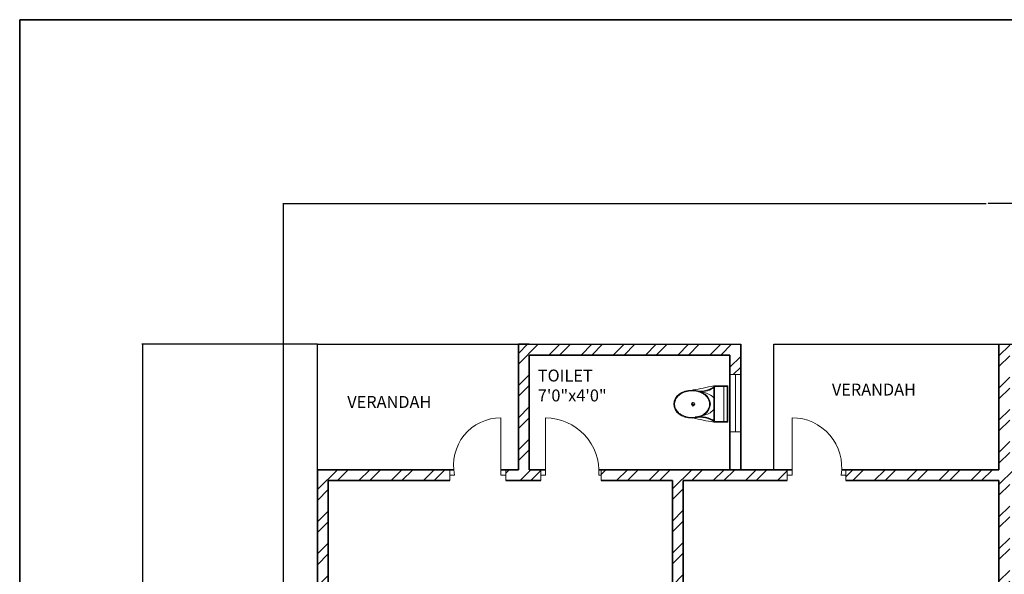
# Model space of a CAD drawing. Units: inches. Extents: x 1962 to 2771, y 1245 to 2660.
# Tile 109 of 114: x 1962 to 2374, y 2428 to 2660. Entities that reach past the tile are written whole.
import ezdxf

# ---------------------------------------------------------------- set-up
doc = ezdxf.new("R2010")
doc.units = ezdxf.units.IN
for name, color, linetype, lineweight in [('A-ANNO-DIMS', 2, 'Continuous', 18), ('A-ANNO-TTLB', 7, 'Continuous', 35), ('A-AREA-IDEN', 7, 'Continuous', 18), ('A-DOOR', 3, 'Continuous', 18), ('A-FLOR-BALC', 7, 'Continuous', 25), ('A-FLOR-FIXT', 8, 'Continuous', 18), ('A-GLAZ', 4, 'Continuous', 18), ('A-WALL', 7, 'Continuous', 35), ('A-WALL-PATT', 252, 'Continuous', 13)]:
    doc.layers.add(name, color=color, linetype=linetype, lineweight=lineweight)
doc.styles.get("Standard").update_dxf_attribs({"font": 'arial.ttf'})
doc.dimstyles.get("Standard").update_dxf_attribs({"dimtxt": 0.18, "dimasz": 0.18, "dimexe": 0.18, "dimexo": 0.0625, "dimgap": 0.09, "dimtad": 0, "dimtih": 1, "dimtoh": 1, "dimdec": 4, "dimzin": 0, "dimdsep": 46, "dimtxsty": 'Standard', "dimcen": 0.09, "dimadec": 0, "dimazin": 0, "dimtfac": 1, "dimtdec": 4, "dimtofl": 0, "dimtmove": 0, "dimatfit": 3, "dimfxl": 1, "dimtolj": 1, "dimtzin": 0, "dimarcsym": 0})

# ---------------------------------------------------------------- blocks, each defined once
blk = doc.blocks.new('A$C31115884')
for p, q in [((283, 498), (223, 498)), ((258, 466), (258, 523)), ((0, 200), (0, 0)), ((520, 200), (0, 200)), ((10, 190), (10, 10)), ((510, 190), (10, 190)), ((510, 10), (510, 190)), ((520, 0), (520, 200)), ((510, 54), (0, 54)), ((10, 10), (510, 10)), ((0, 0), (520, 0))]:
    blk.add_line(p, q)
blk.add_circle((256, 496), 23.6)
for centre, radius, start, end in [((2778, -205), 2807, 165.4549, 171.7133), ((-295, 403), 365, 324.2091, 9.3499), ((-295, 403), 375, 324.2091, 9.3499), ((806, 403), 365, 170.6501, 215.7909), ((3237, 905), 2807, 188.2867, 194.5451), ((384, 406), 293, 190.2774, 224.1564), ((139, 406), 293, 315.8436, 2.6563), ((806, 403), 375, 179.2036, 215.7909)]:
    blk.add_arc(centre, radius, start, end)
blk.add_ellipse((256, 510), major_axis=(0, -261), ratio=0.772727)
blk.add_open_spline([(256, 259), (263, 259), (270, 260), (288, 262), (299, 265), (320, 273), (330, 278), (350, 291), (360, 299), (378, 316), (386, 326), (402, 347), (409, 358), (421, 383), (427, 395), (436, 422), (440, 436), (445, 465), (447, 480), (448, 509), (448, 524), (445, 553), (443, 568), (436, 596), (432, 610), (422, 636), (416, 649), (402, 672), (395, 683), (379, 703), (370, 712), (351, 728), (341, 735), (321, 746), (310, 751), (289, 757), (278, 759), (256, 761), (245, 761), (223, 757), (212, 754), (191, 746), (181, 741), (161, 728), (151, 720), (133, 703), (125, 693), (110, 672), (103, 660), (90, 636), (85, 623), (76, 596), (72, 582), (67, 553), (66, 538), (64, 509), (65, 494), (68, 465), (70, 450), (77, 422), (81, 408), (91, 382), (97, 370), (111, 346), (118, 335), (135, 316), (144, 307), (162, 291), (172, 284), (193, 273), (203, 269), (225, 262), (236, 260), (250, 259), (253, 259), (256, 259)], degree=3, knots=[0, 0, 0, 0, 0.110105, 0.110105, 0.285049, 0.285049, 0.459994, 0.459994, 0.634938, 0.634938, 0.809882, 0.809882, 0.984827, 0.984827, 1.159771, 1.159771, 1.334715, 1.334715, 1.50966, 1.50966, 1.684604, 1.684604, 1.859549, 1.859549, 2.034493, 2.034493, 2.209437, 2.209437, 2.384382, 2.384382, 2.559326, 2.559326, 2.73427, 2.73427, 2.909215, 2.909215, 3.084159, 3.084159, 3.259103, 3.259103, 3.434048, 3.434048, 3.608992, 3.608992, 3.783936, 3.783936, 3.958881, 3.958881, 4.133825, 4.133825, 4.30877, 4.30877, 4.483714, 4.483714, 4.658658, 4.658658, 4.833603, 4.833603, 5.008547, 5.008547, 5.183491, 5.183491, 5.358436, 5.358436, 5.53338, 5.53338, 5.708324, 5.708324, 5.883269, 5.883269, 6.058213, 6.058213, 6.233158, 6.233158, 6.283185, 6.283185, 6.283185, 6.283185])
blk = doc.blocks.new('WIN-24IN-B')
for p, q in [((0, 24), (4.5, 24)), ((4.5, 24), (2.25, 24)), ((2.25, 24), (2.25, 0)), ((4.5, 0), (0, 0)), ((2.25, 0), (4.5, 0))]:
    blk.add_line(p, q)
blk = doc.blocks.new('*D40')
at = {"layer": 'A-ANNO-DIMS', "color": 0, "lineweight": -2, "transparency": 16777216}
for p, q in [((2072.02, 2033.91), (2072.02, 2583.47)), ((2072.2, 2583.29), (2366.02, 2583.29)), ((2660.63, 2583.29), (2366.81, 2583.29)), ((2660.81, 2524.41), (2660.81, 2583.47))]:
    blk.add_line(p, q, dxfattribs=at)
at = {"layer": 'A-ANNO-DIMS', "color": 0, "transparency": 16777216}
for points in [[(2072.2, 2583.32), (2072.2, 2583.26), (2072.02, 2583.29)], [(2660.63, 2583.32), (2660.63, 2583.26), (2660.81, 2583.29)]]:
    blk.add_solid(points, dxfattribs=at)
at = {"layer": 'Defpoints', "color": 0, "transparency": 16777216}
for p in [(2660.81, 2583.29), (2660.81, 2524.34), (2072.02, 2033.84)]:
    blk.add_point(p, dxfattribs=at)
at = {"layer": 'A-ANNO-DIMS', "color": 0, "transparency": 16777216, "insert": (2366.41, 2583.29), "char_height": 0.18, "attachment_point": 5}
blk.add_mtext('\\A1;588.8', dxfattribs=at)
blk = doc.blocks.new('*D43')
at = {"layer": 'A-ANNO-DIMS', "color": 0, "lineweight": -2, "transparency": 16777216}
for p, q in [((2086.24, 2524.34), (2012.89, 2524.34)), ((2013.07, 2524.16), (2013.07, 2279.28)), ((2013.07, 2034.02), (2013.07, 2278.91)), ((2071.96, 2033.84), (2012.89, 2033.84))]:
    blk.add_line(p, q, dxfattribs=at)
at = {"layer": 'A-ANNO-DIMS', "color": 0, "transparency": 16777216}
for points in [[(2013.04, 2524.16), (2013.1, 2524.16), (2013.07, 2524.34)], [(2013.04, 2034.02), (2013.1, 2034.02), (2013.07, 2033.84)]]:
    blk.add_solid(points, dxfattribs=at)
at = {"layer": 'Defpoints', "color": 0, "transparency": 16777216}
for p in [(2086.31, 2524.34), (2013.07, 2033.84), (2072.02, 2033.84)]:
    blk.add_point(p, dxfattribs=at)
at = {"layer": 'A-ANNO-DIMS', "color": 0, "transparency": 16777216, "insert": (2013.07, 2279.09), "char_height": 0.18, "attachment_point": 5}
blk.add_mtext('\\A1;490.5', dxfattribs=at)

msp = doc.modelspace()

# ---------------------------------------------------------------- hatches: boundary and pattern name
at = {"layer": 'A-WALL-PATT'}
h = msp.add_hatch(dxfattribs=at)
h.set_pattern_fill('ANSI32', color=256)
h.paths.add_polyline_path([(2090.8074, 2467.3437), (2141.6481, 2467.3437), (2141.6481, 2469.5937), (2141.6481, 2471.8437), (2086.3074, 2471.8437), (2086.3074, 2422.5333), (2090.8074, 2422.5333)])
h.paths.add_polyline_path([(2282.7664, 2471.8437), (2204.8982, 2471.8437), (2204.8982, 2467.3437), (2234.8074, 2467.3437), (2234.8074, 2311.3437), (2228.7492, 2311.3437), (2228.7492, 2306.8437), (2234.8074, 2306.8437), (2331.9227, 2306.8437), (2331.9227, 2309.0937), (2331.9227, 2311.3437), (2239.3074, 2311.3437), (2239.3074, 2467.3437), (2282.7664, 2467.3437), (2282.7664, 2469.5937)])
h.paths.add_polyline_path([(2471.4531, 2519.8437), (2552.011, 2519.8437), (2564.3996, 2519.8437), (2564.3996, 2511.1389), (2568.8996, 2511.1389), (2568.8996, 2524.3437), (2466.9531, 2524.3437), (2466.9531, 2471.8437), (2450.0749, 2471.8437), (2446.4672, 2471.8437), (2446.4672, 2467.3437), (2450.0749, 2467.3437), (2475.9988, 2467.3437), (2475.9988, 2469.5937), (2475.9988, 2471.8437), (2471.4531, 2471.8437)])
h.paths.add_polyline_path([(2575.2231, 2469.5937), (2575.2231, 2471.8437), (2568.8996, 2471.8437), (2568.8996, 2487.1389), (2564.3996, 2487.1389), (2564.3996, 2471.8437), (2556.511, 2471.8437), (2499.2904, 2471.8437), (2499.2904, 2467.3437), (2507.8074, 2467.3437), (2507.8074, 2311.3437), (2414.863, 2311.3437), (2414.863, 2306.8437), (2512.3074, 2306.8437), (2517.0114, 2306.8437), (2517.0114, 2309.0937), (2517.0114, 2311.3437), (2512.3074, 2311.3437), (2512.3074, 2467.3437), (2575.2231, 2467.3437)])
h.paths.add_polyline_path([(2660.8074, 2471.8437), (2600.9602, 2471.8437), (2600.9602, 2467.3437), (2656.3074, 2467.3437), (2656.3074, 2432.5704), (2660.8074, 2432.5704)])
h.paths.add_polyline_path([(2660.8074, 2372.5704), (2656.3074, 2372.5704), (2656.3074, 2311.3437), (2600.276, 2311.3437), (2600.276, 2309.0937), (2600.276, 2306.8437), (2656.3074, 2306.8437), (2656.3074, 2296.2593), (2660.8074, 2296.2593)])
h.paths.add_polyline_path([(2572.3074, 2306.8437), (2577.1385, 2306.8437), (2577.1385, 2311.3437), (2551.082, 2311.3437), (2551.082, 2306.8437), (2567.8074, 2306.8437), (2567.8074, 2258.8437), (2540.0574, 2258.8437), (2540.0574, 2256.5937), (2540.0574, 2254.3437), (2567.8074, 2254.3437), (2656.3074, 2254.3437), (2656.3074, 2236.9085), (2660.8074, 2236.9085), (2660.8074, 2272.2593), (2656.3074, 2272.2593), (2656.3074, 2258.8437), (2572.3074, 2258.8437)])
h.paths.add_polyline_path([(2512.3074, 2254.3437), (2518.8716, 2254.3437), (2518.8716, 2256.5937), (2518.8716, 2258.8437), (2507.8074, 2258.8437), (2507.8074, 2177.8437), (2567.8074, 2177.8437), (2567.8074, 2172.9628), (2572.3074, 2172.9628), (2572.3074, 2177.8437), (2656.3074, 2177.8437), (2656.3074, 2166.4846), (2660.8074, 2166.4846), (2660.8074, 2200.9085), (2656.3074, 2200.9085), (2656.3074, 2182.3437), (2512.3074, 2182.3437)])
h.paths.add_polyline_path([(2656.3074, 2129.8437), (2572.3074, 2129.8437), (2572.3074, 2150.3044), (2570.0574, 2150.3044), (2567.8074, 2150.3044), (2567.8074, 2129.8437), (2507.8074, 2129.8437), (2507.8074, 2116.3027), (2510.0574, 2116.3027), (2512.3074, 2116.3027), (2512.3074, 2125.3437), (2567.8074, 2125.3437), (2572.3074, 2125.3437), (2656.3074, 2125.3437)])
h.paths.add_polyline_path([(2090.8074, 2362.5333), (2086.3074, 2362.5333), (2086.3074, 2298.6242), (2090.8074, 2298.6242), (2090.8074, 2306.8437), (2174.8074, 2306.8437), (2174.8074, 2286.4178), (2179.3074, 2286.4178), (2179.3074, 2306.8437), (2192.8641, 2306.8437), (2192.8641, 2309.0937), (2192.8641, 2311.3437), (2090.8074, 2311.3437)])
h.paths.add_polyline_path([(2209.156, 2258.8437), (2179.3074, 2258.8437), (2179.3074, 2263.2236), (2177.0574, 2263.2236), (2174.8074, 2263.2236), (2174.8074, 2258.8437), (2090.8074, 2258.8437), (2090.8074, 2274.6242), (2086.3074, 2274.6242), (2086.3074, 2238.2967), (2088.5574, 2238.2967), (2090.8074, 2238.2967), (2090.8074, 2254.3437), (2209.156, 2254.3437)])
h.paths.add_polyline_path([(2090.8074, 2177.8437), (2234.8074, 2177.8437), (2234.8074, 2173.1428), (2239.3074, 2173.1428), (2239.3074, 2258.8437), (2230.8442, 2258.8437), (2230.8442, 2256.5937), (2230.8442, 2254.3437), (2234.8074, 2254.3437), (2234.8074, 2182.3437), (2090.8074, 2182.3437), (2090.8074, 2202.2967), (2086.3074, 2202.2967), (2086.3074, 2140.0389), (2090.8074, 2140.0389)])
h.paths.add_polyline_path([(2090.8074, 2080.0389), (2086.3074, 2080.0389), (2086.3074, 2033.8437), (2090.8074, 2033.8437)], flags=17)
h.paths.add_polyline_path([(2244.9405, 2033.8437), (2239.3074, 2033.8437), (2239.3074, 2142.0665), (2237.2592, 2142.0665), (2234.8074, 2142.0665), (2234.8074, 2033.8437), (2090.8074, 2033.8437), (2076.5204, 2033.8437), (2072.0204, 2033.8437), (2072.0204, 2000.4493), (2076.5204, 2000.4493), (2076.5204, 2029.3437), (2090.8074, 2029.3437), (2244.9405, 2029.3437), (2244.9405, 2031.5937)])
h.paths.add_polyline_path([(2234.8074, 1933.3437), (2076.5204, 1933.3437), (2076.5204, 1952.4493), (2074.2704, 1952.4493), (2072.0204, 1952.4493), (2072.0204, 1933.3437), (2072.0204, 1928.8437), (2234.8074, 1928.8437)])
h.paths.add_polyline_path([(2090.8074, 1928.8437), (2086.3074, 1928.8437), (2086.3074, 1906.5013), (2090.8074, 1906.5013)])
h.paths.add_polyline_path([(2090.8074, 1846.5013), (2086.3074, 1846.5013), (2086.3074, 1769.9917), (2088.5574, 1769.9917), (2090.8074, 1769.9917), (2090.8074, 1780.3437), (2234.8074, 1780.3437), (2234.8074, 1708.3437), (2230.3764, 1708.3437), (2230.3764, 1703.8437), (2239.3074, 1703.8437), (2239.3074, 1792.6669), (2237.0574, 1792.6669), (2234.8074, 1792.6669), (2234.8074, 1784.8437), (2090.8074, 1784.8437)])
h.paths.add_polyline_path([(2239.3074, 1928.8437), (2244.9405, 1928.8437), (2244.9405, 1931.0937), (2244.9405, 1933.3437), (2234.8074, 1933.3437), (2234.8074, 1928.8437), (2234.8074, 1825.5949), (2239.3074, 1825.5949)])
h.paths.add_polyline_path([(2148.0425, 1649.0937), (2148.0425, 1651.3437), (2090.8074, 1651.3437), (2090.8074, 1646.8437), (2148.0425, 1646.8437)], flags=0)
h.paths.add_polyline_path([(2207.5601, 1708.3437), (2090.8074, 1708.3437), (2090.8074, 1703.8437), (2174.8074, 1703.8437), (2174.8074, 1651.3437), (2170.4457, 1651.3437), (2170.4457, 1646.8437), (2195.9924, 1646.8437), (2195.9924, 1649.0937), (2195.9924, 1651.3437), (2179.3074, 1651.3437), (2179.3074, 1703.8437), (2207.5601, 1703.8437), (2207.5601, 1706.0937)])
h.paths.add_polyline_path([(2090.8074, 1733.9917), (2086.3074, 1733.9917), (2086.3074, 1696.1032), (2088.5574, 1696.1032), (2090.8074, 1696.1032)])
h.paths.add_polyline_path([(2090.8074, 1672.1032), (2086.3074, 1672.1032), (2086.3074, 1600.3335), (2090.8074, 1600.3335)])
h.paths.add_polyline_path([(2090.8074, 1540.3335), (2086.3074, 1540.3335), (2086.3074, 1486.3437), (2139.6766, 1486.3437), (2139.6766, 1490.8437), (2090.8074, 1490.8437)])
h.paths.add_polyline_path([(2302.3876, 1490.8437), (2239.3074, 1490.8437), (2239.3074, 1646.8437), (2335.9994, 1646.8437), (2335.9994, 1651.3437), (2229.884, 1651.3437), (2229.884, 1646.8437), (2234.8074, 1646.8437), (2234.8074, 1490.8437), (2202.7103, 1490.8437), (2202.7103, 1488.5937), (2202.7103, 1486.3437), (2275.0699, 1486.3437), (2275.0699, 1475.772), (2279.5699, 1475.772), (2279.5699, 1486.3437), (2302.3876, 1486.3437)])
h.paths.add_polyline_path([(2279.5699, 1451.772), (2275.0699, 1451.772), (2275.0699, 1438.3437), (2174.8074, 1438.3437), (2174.8074, 1486.3437), (2179.7922, 1486.3437), (2179.7922, 1490.8437), (2163.3585, 1490.8437), (2163.3585, 1488.5937), (2163.3585, 1486.3437), (2170.3074, 1486.3437), (2170.3074, 1433.8437), (2279.5699, 1433.8437)])
h.paths.add_polyline_path([(2427.2363, 1490.8437), (2375.8074, 1490.8437), (2375.8074, 1646.8437), (2381.6401, 1646.8437), (2381.6401, 1651.3437), (2365.887, 1651.3437), (2365.887, 1649.0937), (2365.887, 1646.8437), (2371.3074, 1646.8437), (2371.3074, 1490.8437), (2327.5627, 1490.8437), (2327.5627, 1488.5937), (2327.5627, 1486.3437), (2371.3074, 1486.3437), (2371.3074, 1433.8437), (2375.8074, 1433.8437), (2375.8074, 1486.3437), (2427.2363, 1486.3437)])
h.paths.add_polyline_path([(2512.3074, 1646.8437), (2519.4351, 1646.8437), (2519.4351, 1649.0937), (2519.4351, 1651.3437), (2507.8074, 1651.3437), (2416.0063, 1651.3437), (2416.0063, 1649.0937), (2416.0063, 1646.8437), (2507.8074, 1646.8437), (2507.8074, 1490.8437), (2497.0532, 1490.8437), (2497.0532, 1488.5937), (2497.0532, 1486.3437), (2574.9344, 1486.3437), (2574.9344, 1476.0181), (2579.4344, 1476.0181), (2579.4344, 1486.3437), (2584.4872, 1486.3437), (2584.3074, 1490.8437), (2512.3074, 1490.8437)])
h.paths.add_polyline_path([(2470.5091, 1486.3437), (2473.9767, 1486.3437), (2473.9767, 1490.8437), (2449.6605, 1490.8437), (2449.6605, 1488.5937), (2449.6605, 1486.3437), (2466.0091, 1486.3437), (2466.0091, 1433.8437), (2470.5091, 1433.8437), (2579.4344, 1433.8437), (2579.4344, 1452.0181), (2574.9344, 1452.0181), (2574.9344, 1438.3437), (2554.5091, 1438.3437), (2470.5091, 1438.3437)])
h.paths.add_polyline_path([(2656.3074, 1490.8437), (2611.86, 1490.8437), (2611.86, 1486.3437), (2656.3074, 1486.3437)])
h.paths.add_polyline_path([(2660.8074, 1532.7007), (2658.5574, 1532.7007), (2656.3074, 1532.7007), (2656.3074, 1486.3437), (2660.8074, 1486.3437)])
h.paths.add_polyline_path([(2660.8074, 1664.9663), (2656.3074, 1664.9663), (2656.3074, 1651.3437), (2602.2313, 1651.3437), (2602.2313, 1646.8437), (2656.3074, 1646.8437), (2656.3074, 1592.7007), (2660.8074, 1592.7007)])
h.paths.add_polyline_path([(2660.8074, 1724.5221), (2656.3074, 1724.5221), (2656.3074, 1703.8437), (2542.4725, 1703.8437), (2542.4725, 1699.3437), (2567.8074, 1699.3437), (2567.8074, 1651.3437), (2552.7766, 1651.3437), (2552.7766, 1649.0937), (2552.7766, 1646.8437), (2577.2878, 1646.8437), (2577.2878, 1649.0937), (2577.2878, 1651.3437), (2572.3074, 1651.3437), (2572.3074, 1699.3437), (2656.3074, 1699.3437), (2656.3074, 1688.9663), (2660.8074, 1688.9663)])
h.paths.add_polyline_path([(2660.8074, 1880.6524), (2656.3074, 1880.6524), (2656.3074, 1832.8437), (2512.3074, 1832.8437), (2512.3074, 1837.8959), (2507.8074, 1837.8959), (2507.8074, 1828.3437), (2567.8074, 1828.3437), (2567.8074, 1804.3437), (2572.3074, 1804.3437), (2572.3074, 1828.3437), (2656.3074, 1828.3437), (2656.3074, 1818.6778), (2660.8074, 1818.6778)])
h.paths.add_polyline_path([(2660.8074, 1794.6778), (2656.3074, 1794.6778), (2656.3074, 1780.3437), (2572.3074, 1780.3437), (2572.3074, 1783.0303), (2570.0574, 1783.0303), (2567.8074, 1783.0303), (2567.8074, 1780.3437), (2507.8074, 1780.3437), (2507.8074, 1699.3437), (2517.8858, 1699.3437), (2517.8858, 1701.5937), (2517.8858, 1703.8437), (2512.3074, 1703.8437), (2512.3074, 1775.8437), (2656.3074, 1775.8437), (2656.3074, 1760.5221), (2660.8074, 1760.5221)])
h.paths.add_polyline_path([(2660.8074, 1981.3437), (2660.8074, 2020.2808), (2658.5574, 2020.2808), (2656.3074, 2020.2808), (2656.3074, 1981.3437), (2512.3074, 1981.3437), (2512.3074, 2086.6996), (2507.8074, 2086.6996), (2507.8074, 1981.3437), (2375.8074, 1981.3437), (2375.8074, 1986.8505), (2373.5574, 1986.8505), (2371.3074, 1986.8505), (2371.3074, 1973.2607), (2375.8074, 1973.2607), (2375.8074, 1976.8437), (2507.8074, 1976.8437), (2507.8074, 1865.4281), (2510.0574, 1865.4281), (2512.3074, 1865.4281), (2512.3074, 1976.8437), (2660.8074, 1976.8437)])
h.paths.add_polyline_path([(2375.8074, 1940.297), (2373.5574, 1940.297), (2371.3074, 1940.297), (2371.3074, 1933.3437), (2278.4434, 1933.3437), (2278.4434, 1928.8437), (2371.3074, 1928.8437), (2371.3074, 1651.3437), (2375.8074, 1651.3437)])
h.paths.add_polyline_path([(2660.8074, 1976.8437), (2656.3074, 1976.8437), (2656.3074, 1940.6524), (2660.8074, 1940.6524)], flags=17)
h.paths.add_polyline_path([(2660.8074, 2142.4846), (2656.3074, 2142.4846), (2656.3074, 2080.2808), (2660.8074, 2080.2808)])
h.paths.add_polyline_path([(2381.4189, 2311.3437), (2375.8074, 2311.3437), (2375.8074, 2467.3437), (2424.7242, 2467.3437), (2424.7242, 2469.5937), (2424.7242, 2471.8437), (2375.8074, 2471.8437), (2375.8074, 2524.3437), (2371.3074, 2524.3437), (2371.3074, 2471.8437), (2307.2097, 2471.8437), (2307.2097, 2467.3437), (2371.3074, 2467.3437), (2371.3074, 2311.3437), (2366.8901, 2311.3437), (2366.8901, 2306.8437), (2371.3074, 2306.8437), (2371.3074, 2033.8437), (2279.6589, 2033.8437), (2279.6589, 2029.3437), (2371.3074, 2029.3437), (2371.3074, 2014.2598), (2375.8074, 2014.2598), (2375.8074, 2306.8437), (2381.4189, 2306.8437)])
h.paths.add_polyline_path([(2263.3074, 2524.3437), (2170.3074, 2524.3437), (2170.3074, 2519.8437), (2170.3074, 2471.8437), (2165.0312, 2471.8437), (2165.0312, 2467.3437), (2179.6721, 2467.3437), (2179.6721, 2469.5161), (2179.6721, 2471.8437), (2174.8074, 2471.8437), (2174.8074, 2519.8437), (2258.8074, 2519.8437), (2258.8074, 2511.6436), (2263.3074, 2511.6436)])
h.paths.add_polyline_path([(2245.0232, 1361.4123), (2492.9468, 1361.4123), (2492.9468, 1398.505), (2245.0232, 1398.505)], flags=9)
h.paths.add_polyline_path([(2388.1434, 2086.6936), (2425.0704, 2086.6936), (2425.0704, 2105.3509), (2388.1434, 2105.3509)], flags=9)
h.paths.add_polyline_path([(2404.922, 2242.6744), (2445.7337, 2242.6744), (2445.7337, 2261.3318), (2404.922, 2261.3318)], flags=9)
h.paths.add_polyline_path([(2269.4107, 2156.7935), (2306.3378, 2156.7935), (2306.3378, 2175.4508), (2269.4107, 2175.4508)], flags=9)
h.paths.add_polyline_path([(2269.3277, 2233.4343), (2306.2547, 2233.4343), (2306.2547, 2252.0917), (2269.3277, 2252.0917)], flags=9)
h.paths.add_polyline_path([(2431.6052, 2320.6922), (2470.4456, 2320.6922), (2470.4456, 2339.3495), (2431.6052, 2339.3495)], flags=25)
h.paths.add_polyline_path([(2249.6902, 2315.7608), (2288.5306, 2315.7608), (2288.5306, 2334.4182), (2249.6902, 2334.4182)], flags=25)
h.paths.add_polyline_path([(2096.9301, 2314.3181), (2135.7704, 2314.3181), (2135.7704, 2332.9755), (2096.9301, 2332.9755)], flags=25)
h.paths.add_polyline_path([(2134.3475, 2285.7089), (2161.4655, 2285.7089), (2161.4655, 2304.3662), (2134.3475, 2304.3662)], flags=9)
h.paths.add_polyline_path([(2126.5155, 2209.4076), (2159.9227, 2209.4076), (2159.9227, 2228.065), (2126.5155, 2228.065)], flags=25)
h.paths.add_polyline_path([(2110.5753, 2141.5299), (2149.4157, 2141.5299), (2149.4157, 2160.1872), (2110.5753, 2160.1872)], flags=25)
h.paths.add_polyline_path([(2249.8618, 1968.3317), (2286.3966, 1968.3317), (2286.3966, 1986.989), (2249.8618, 1986.989)], flags=9)
h.paths.add_polyline_path([(2395.9507, 1777.0051), (2436.7624, 1777.0051), (2436.7624, 1795.6625), (2395.9507, 1795.6625)], flags=9)
h.paths.add_polyline_path([(2398.5259, 1888.5651), (2435.0062, 1888.5651), (2435.0062, 1907.2224), (2398.5259, 1907.2224)], flags=25)
h.paths.add_polyline_path([(2259.3506, 1728.3559), (2296.2776, 1728.3559), (2296.2776, 1747.0132), (2259.3506, 1747.0132)], flags=9)
h.paths.add_polyline_path([(2271.3698, 1845.268), (2308.2968, 1845.268), (2308.2968, 1863.9253), (2271.3698, 1863.9253)], flags=9)
h.paths.add_polyline_path([(2120.9355, 1786.3027), (2159.7759, 1786.3027), (2159.7759, 1804.9601), (2120.9355, 1804.9601)], flags=25)
h.paths.add_polyline_path([(2121.3164, 1732.1043), (2154.7236, 1732.1043), (2154.7236, 1750.7616), (2121.3164, 1750.7616)], flags=25)
h.paths.add_polyline_path([(2118.3706, 1678.8997), (2147.5282, 1678.8997), (2147.5282, 1697.557), (2118.3706, 1697.557)], flags=25)
h.paths.add_polyline_path([(2385.9227, 1493.557), (2424.763, 1493.557), (2424.763, 1512.2143), (2385.9227, 1512.2143)], flags=25)
h.paths.add_polyline_path([(2248.7058, 1500.0256), (2287.5462, 1500.0256), (2287.5462, 1518.6829), (2248.7058, 1518.6829)], flags=25)
h.paths.add_polyline_path([(2104.1669, 1617.3771), (2143.0073, 1617.3771), (2143.0073, 1636.0344), (2104.1669, 1636.0344)], flags=9)
h.paths.add_polyline_path([(2096.0714, 1447.8824), (2137.3845, 1447.8824), (2137.3845, 1458.1859), (2096.0714, 1458.1859)], flags=9)
h.paths.add_polyline_path([(2180.6114, 1440.325), (2209.7689, 1440.325), (2209.7689, 1458.9823), (2180.6114, 1458.9823)], flags=25)
h.paths.add_polyline_path([(2316.1698, 1447.9637), (2357.4829, 1447.9637), (2357.4829, 1458.2673), (2316.1698, 1458.2673)], flags=9)
h.paths.add_polyline_path([(2397.6187, 1447.9637), (2438.9318, 1447.9637), (2438.9318, 1458.2673), (2397.6187, 1458.2673)], flags=9)
h.paths.add_polyline_path([(2473.0778, 1439.5953), (2502.2354, 1439.5953), (2502.2354, 1458.2527), (2473.0778, 1458.2527)], flags=25)
h.paths.add_polyline_path([(2589.7027, 1447.8819), (2631.0158, 1447.8819), (2631.0158, 1458.1855), (2589.7027, 1458.1855)], flags=9)
h.paths.add_polyline_path([(2522.4009, 1497.5285), (2561.2413, 1497.5285), (2561.2413, 1516.1859), (2522.4009, 1516.1859)], flags=25)
h.paths.add_polyline_path([(2579.6565, 1671.3482), (2608.8141, 1671.3482), (2608.8141, 1690.0056), (2579.6565, 1690.0056)], flags=25)
h.paths.add_polyline_path([(2544.7038, 1725.5064), (2578.1111, 1725.5064), (2578.1111, 1744.1637), (2544.7038, 1744.1637)], flags=25)
h.paths.add_polyline_path([(2578.1191, 1807.472), (2607.2766, 1807.472), (2607.2766, 1826.1293), (2578.1191, 1826.1293)], flags=25)
h.paths.add_polyline_path([(2595.0614, 1835.1839), (2633.9018, 1835.1839), (2633.9018, 1853.8413), (2595.0614, 1853.8413)], flags=25)
h.paths.add_polyline_path([(2567.0097, 2097.7035), (2605.8501, 2097.7035), (2605.8501, 2116.3609), (2567.0097, 2116.3609)], flags=9)
h.paths.add_polyline_path([(2586.644, 2134.6454), (2615.8015, 2134.6454), (2615.8015, 2153.3027), (2586.644, 2153.3027)], flags=9)
h.paths.add_polyline_path([(2544.6185, 2212.6783), (2578.0258, 2212.6783), (2578.0258, 2231.3356), (2544.6185, 2231.3356)], flags=25)
h.paths.add_polyline_path([(2577.0273, 2256.9023), (2606.1849, 2256.9023), (2606.1849, 2275.5597), (2577.0273, 2275.5597)], flags=24)
h.paths.add_polyline_path([(2605.2683, 2315.2821), (2644.1087, 2315.2821), (2644.1087, 2333.9395), (2605.2683, 2333.9395)], flags=25)
h.paths.add_polyline_path([(2583.1244, 2496.1815), (2624.4375, 2496.1815), (2624.4375, 2506.4851), (2583.1244, 2506.4851)], flags=9)
h.paths.add_polyline_path([(2474.761, 2497.0823), (2503.9185, 2497.0823), (2503.9185, 2515.7397), (2474.761, 2515.7397)], flags=25)
h.paths.add_polyline_path([(2387.5787, 2494.2563), (2428.902, 2494.2563), (2428.902, 2504.5598), (2387.5787, 2504.5598)], flags=9)
h.paths.add_polyline_path([(2300.1657, 2500.1564), (2341.4788, 2500.1564), (2341.4788, 2510.46), (2300.1657, 2510.46)], flags=25)
h.paths.add_polyline_path([(2176.8589, 2497.5843), (2206.0165, 2497.5843), (2206.0165, 2516.2416), (2176.8589, 2516.2416)], flags=25)
h.paths.add_polyline_path([(2097.4668, 2494.9762), (2138.7799, 2494.9762), (2138.7799, 2505.2798), (2097.4668, 2505.2798)], flags=9)

# ---------------------------------------------------------------- linework, layer by layer
at = {"layer": 'A-ANNO-TTLB'}
msp.add_lwpolyline([(1961.7365, 2660.2579), (2771.213, 2660.2579), (2771.213, 1244.5817), (1961.7365, 1244.5817)], close=True, dxfattribs=at)
at = {"layer": 'A-DOOR'}
for p, q in [((2163.0312, 2469.5937), (2163.0312, 2493.5937)), ((2181.6721, 2469.5161), (2181.6721, 2493.5161)), ((2284.7664, 2469.5937), (2284.7664, 2493.5937)), ((2141.6481, 2471.8437), (2141.6481, 2467.3437)), ((2165.0312, 2471.8437), (2165.0312, 2467.3437)), ((2179.6721, 2471.8437), (2179.6721, 2468.4349)), ((2204.8982, 2471.8437), (2204.8982, 2467.3437)), ((2282.7664, 2471.8437), (2282.7664, 2467.3437)), ((2307.2097, 2471.8437), (2307.2097, 2467.3437)), ((2141.6481, 2467.3437), (2141.6481, 2469.5937)), ((2141.6481, 2469.5937), (2143.6481, 2469.5937)), ((2165.0312, 2469.5937), (2163.0312, 2469.5937)), ((2165.0312, 2467.3437), (2165.0312, 2469.5937)), ((2179.6721, 2467.3437), (2179.6721, 2469.5161)), ((2179.6721, 2469.5161), (2181.6721, 2469.5161)), ((2179.6721, 2468.4349), (2179.6721, 2467.3437)), ((2204.8982, 2469.5937), (2203.8982, 2469.5937)), ((2204.8982, 2467.3437), (2204.8982, 2469.5937)), ((2282.7664, 2467.3437), (2282.7664, 2469.5937)), ((2282.7664, 2469.5937), (2284.7664, 2469.5937)), ((2307.2097, 2469.5937), (2305.2097, 2469.5937)), ((2307.2097, 2467.3437), (2307.2097, 2469.5937))]:
    msp.add_line(p, q, dxfattribs=at)
for centre, radius, start, end in [((2163.0312, 2473.7665), 19.8272, 90, 192.149314), ((2181.6721, 2471.2299), 22.2862, 355.7897, 90), ((2284.7664, 2472.8034), 20.7903, 351.118747, 90)]:
    msp.add_arc(centre, radius, start, end, dxfattribs=at)
at = {"layer": 'A-FLOR-BALC'}
for p, q in [((2086.3074, 2519.8437), (2086.3074, 2524.3437)), ((2086.3074, 2524.3437), (2263.3074, 2524.3437)), ((2277.2053, 2471.8437), (2277.2053, 2524.3437)), ((2277.2053, 2524.3437), (2370.0887, 2524.3437)), ((2277.2053, 2524.3437), (2450.0749, 2524.3437)), ((2086.3074, 2471.8437), (2086.3074, 2519.8437))]:
    msp.add_line(p, q, dxfattribs=at)
at = {"layer": 'A-WALL'}
for p, q in [((2170.3074, 2471.8437), (2170.3074, 2524.3437)), ((2170.3074, 2524.3437), (2174.8074, 2524.3437)), ((2170.3074, 2524.3437), (2170.3074, 2519.8437)), ((2263.3074, 2471.8437), (2263.3074, 2524.3437)), ((2371.3074, 2471.8437), (2371.3074, 2524.3437)), ((2174.8074, 2519.8437), (2174.8074, 2471.8437)), ((2174.8074, 2519.8437), (2258.8074, 2519.8437)), ((2258.8074, 2519.8437), (2258.8074, 2471.8437)), ((2086.3074, 2471.8437), (2143.2975, 2471.8437)), ((2086.3074, 2471.8437), (2086.3074, 2033.8437)), ((2086.3074, 2471.8437), (2143.2975, 2471.8437)), ((2163.0312, 2471.8437), (2170.3074, 2471.8437)), ((2163.0312, 2471.8437), (2170.3074, 2471.8437)), ((2174.8074, 2471.8437), (2181.6721, 2471.8437)), ((2203.9499, 2471.8437), (2284.7664, 2471.8437)), ((2258.8074, 2471.8437), (2263.3074, 2471.8437)), ((2305.5345, 2471.8437), (2371.3074, 2471.8437)), ((2090.8074, 2467.3437), (2141.6481, 2467.3437)), ((2090.8074, 2467.3437), (2090.8074, 2311.3437)), ((2165.0312, 2467.3437), (2179.6721, 2467.3437)), ((2204.8982, 2467.3437), (2234.8074, 2467.3437)), ((2234.8074, 2467.3437), (2234.8074, 2311.3437)), ((2239.3074, 2467.3437), (2239.3074, 2311.3437)), ((2239.3074, 2467.3437), (2282.7664, 2467.3437)), ((2307.2097, 2467.3437), (2371.3074, 2467.3437)), ((2371.3074, 2467.3437), (2371.3074, 2311.3437))]:
    msp.add_line(p, q, dxfattribs=at)

# ---------------------------------------------------------------- block references
at = {"layer": 'A-FLOR-FIXT', "xscale": 0.0292470664339069, "yscale": 0.0292470664339069, "zscale": 0.0292470664339069, "rotation": 89.99999999999999}
msp.add_blockref('A$C31115884', (2257.8905, 2491.786), dxfattribs=at)
at = {"layer": 'A-GLAZ'}
msp.add_blockref('WIN-24IN-B', (2258.8074, 2487.6436), dxfattribs=at)

# ---------------------------------------------------------------- texts
at = {"layer": 'A-AREA-IDEN', "char_height": 5, "attachment_point": 1}
for s, width, insert in [('TOILET\\P7\'0"x4\'0"', 72.02479, (2178.4397, 2513.757)), ('VERANDAH', 90.748727, (2301.4464, 2507.8866)), ('VERANDAH', 222.900056, (2098.7475, 2502.7064))]:
    msp.add_mtext_dynamic_manual_height_columns(s, width=width, gutter_width=12.5, heights=[0], dxfattribs=dict(at, insert=insert))

# ---------------------------------------------------------------- dimensions: what is measured, and where the dimension line sits
at = {"layer": 'A-ANNO-DIMS'}
dim = msp.add_linear_dim(base=(2660.8074, 2583.2937), p1=(2072.0204, 2033.8437), p2=(2660.8074, 2524.3437), dimstyle='Standard', override={"dimdec": 1, "dimlfac": 1, "dimrnd": 0, "dimzin": 0, "dimdsep": 46, "dimlunit": 2}, dxfattribs=at)
dim.commit()
dim.dimension.update_dxf_attribs({"geometry": '*D40', "text_midpoint": (2366.4139, 2583.2937)})
dim = msp.add_linear_dim(base=(2013.0704, 2033.8437), p1=(2086.3074, 2524.3437), p2=(2072.0204, 2033.8437), angle=90, dimstyle='Standard', override={"dimdec": 1, "dimlfac": 1, "dimrnd": 0, "dimzin": 0, "dimdsep": 46, "dimlunit": 2}, dxfattribs=at)
dim.commit()
dim.dimension.update_dxf_attribs({"geometry": '*D43', "text_midpoint": (2013.0704, 2279.0937)})

doc.saveas('drawing.dxf')
